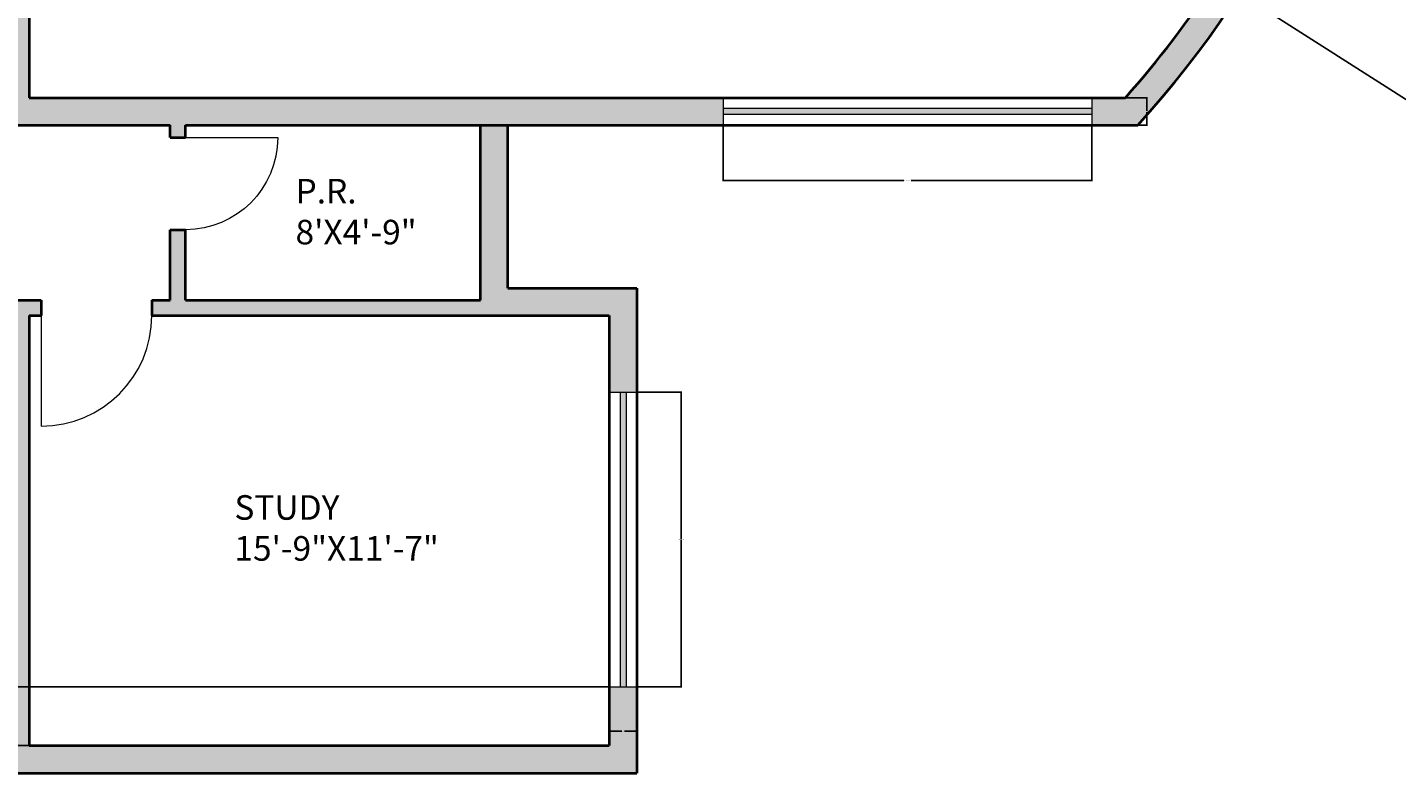
# Model space of a CAD drawing. Units: inches. Extents: x 2330 to 3943, y 1763 to 3461.
# Tile 13 of 40: x 2977 to 3423, y 2300 to 2547. Entities that reach past the tile are written whole.
import ezdxf

# ---------------------------------------------------------------- set-up
doc = ezdxf.new("R2010")
doc.units = ezdxf.units.IN
for name, color, linetype, lineweight in [('A-ANNO-DIMS', 2, 'Continuous', 18), ('A-AREA-IDEN', 7, 'Continuous', 18), ('A-DOOR', 4, 'Continuous', 18), ('A-GLAZ', 4, 'Continuous', 18), ('A-WALL', 7, 'Continuous', 40), ('A-WALL-PATT', 252, 'Continuous', 13), ('L-PLNT', 94, 'Continuous', 13)]:
    doc.layers.add(name, color=color, linetype=linetype, lineweight=lineweight)
doc.styles.get("Standard").update_dxf_attribs({"font": 'arial.ttf'})
doc.dimstyles.get("Standard").update_dxf_attribs({"dimtxt": 0.18, "dimasz": 0.18, "dimexe": 0.18, "dimexo": 0.0625, "dimgap": 0.09, "dimtad": 0, "dimtih": 1, "dimtoh": 1, "dimdec": 4, "dimzin": 0, "dimdsep": 46, "dimtxsty": 'Standard', "dimcen": 0.09, "dimadec": 0, "dimazin": 0, "dimtfac": 1, "dimtdec": 4, "dimtofl": 0, "dimtmove": 0, "dimatfit": 3, "dimfxl": 1, "dimtolj": 1, "dimtzin": 0, "dimarcsym": 0})

# ---------------------------------------------------------------- blocks, each defined once
blk = doc.blocks.new('DOOR-SINGLE-36IN')
blk.add_line((0, 0), (-36, 0))
blk.add_arc((0, 0), 36, 180, 270)
blk = doc.blocks.new('DOOR-SINGLE-30IN')
blk.add_line((0, 0), (0, 30))
blk.add_arc((0, 0), 30, 90, 180)
blk = doc.blocks.new('WINDOW-96IN')
h = blk.add_hatch(color=256)
h.dxf.hatch_style = 1
h.paths.add_polyline_path([(5.5, 96), (3.5, 96), (3.5, 0), (5.5, 0)])
for p, q in [((0, 96), (9, 96)), ((3.5, 96), (3.5, 0)), ((5.5, 96), (5.5, 0)), ((0, 0), (9, 0))]:
    blk.add_line(p, q)
blk = doc.blocks.new('WINDOW-120IN')
h = blk.add_hatch(color=256)
h.dxf.hatch_style = 1
h.paths.add_polyline_path([(120, 5.5), (0, 5.5), (0, 3.5), (120, 3.5)])
for p, q in [((0, 9), (0, 0)), ((120, 9), (120, 0)), ((120, 5.5), (0, 5.5)), ((120, 3.5), (0, 3.5))]:
    blk.add_line(p, q)
blk = doc.blocks.new('*D33')
at = {"layer": 'A-ANNO-DIMS', "color": 0, "lineweight": -2, "transparency": 16777216}
for p, q in [((3203.78, 2514.59), (3203.78, 2496.47)), ((3323.78, 2514.59), (3323.78, 2496.47)), ((3203.96, 2496.65), (3262.59, 2496.65)), ((3323.6, 2496.65), (3264.97, 2496.65))]:
    blk.add_line(p, q, dxfattribs=at)
at = {"layer": 'A-ANNO-DIMS', "color": 0, "transparency": 16777216}
for points in [[(3203.96, 2496.68), (3203.96, 2496.62), (3203.78, 2496.65)], [(3323.6, 2496.68), (3323.6, 2496.62), (3323.78, 2496.65)]]:
    blk.add_solid(points, dxfattribs=at)
at = {"layer": 'Defpoints', "color": 0, "transparency": 16777216}
for p in [(3203.78, 2514.65), (3323.78, 2514.65), (3323.78, 2496.65)]:
    blk.add_point(p, dxfattribs=at)
at = {"layer": 'A-ANNO-DIMS', "color": 0, "transparency": 16777216, "insert": (3263.78, 2496.65), "char_height": 0.18, "attachment_point": 5}
blk.add_mtext('\\A1;WINDOW 120 TYP.', dxfattribs=at)
blk = doc.blocks.new('*D34')
at = {"layer": 'A-ANNO-DIMS', "color": 0, "lineweight": -2, "transparency": 16777216}
for p, q in [((3323.84, 2523.65), (3341.96, 2523.65)), ((3341.78, 2523.47), (3341.78, 2519.33)), ((3341.78, 2514.83), (3341.78, 2518.97)), ((3323.84, 2514.65), (3341.96, 2514.65))]:
    blk.add_line(p, q, dxfattribs=at)
at = {"layer": 'A-ANNO-DIMS', "color": 0, "transparency": 16777216}
for points in [[(3341.75, 2523.47), (3341.81, 2523.47), (3341.78, 2523.65)], [(3341.75, 2514.83), (3341.81, 2514.83), (3341.78, 2514.65)]]:
    blk.add_solid(points, dxfattribs=at)
at = {"layer": 'Defpoints', "color": 0, "transparency": 16777216}
for p in [(3323.78, 2523.65), (3341.78, 2523.65), (3323.78, 2514.65)]:
    blk.add_point(p, dxfattribs=at)
at = {"layer": 'A-ANNO-DIMS', "color": 0, "transparency": 16777216, "insert": (3341.78, 2519.15), "char_height": 0.18, "attachment_point": 5}
blk.add_mtext('\\A1;9 TYP.', dxfattribs=at)
blk = doc.blocks.new('*D35')
at = {"layer": 'A-ANNO-DIMS', "color": 0, "lineweight": -2, "transparency": 16777216}
for p, q in [((3175.72, 2427.7), (3190.24, 2427.7)), ((3190.06, 2427.52), (3190.06, 2379.88)), ((3190.06, 2331.88), (3190.06, 2379.52)), ((3175.72, 2331.7), (3190.24, 2331.7))]:
    blk.add_line(p, q, dxfattribs=at)
at = {"layer": 'A-ANNO-DIMS', "color": 0, "transparency": 16777216}
for points in [[(3190.03, 2427.52), (3190.09, 2427.52), (3190.06, 2427.7)], [(3190.03, 2331.88), (3190.09, 2331.88), (3190.06, 2331.7)]]:
    blk.add_solid(points, dxfattribs=at)
at = {"layer": 'Defpoints', "color": 0, "transparency": 16777216}
for p in [(3175.66, 2427.7), (3190.06, 2427.7), (3175.66, 2331.7)]:
    blk.add_point(p, dxfattribs=at)
at = {"layer": 'A-ANNO-DIMS', "color": 0, "transparency": 16777216, "insert": (3190.06, 2379.7), "char_height": 0.18, "attachment_point": 5}
blk.add_mtext('\\A1;WINDOW 96 TYP.', dxfattribs=at)
blk = doc.blocks.new('*D36')
at = {"layer": 'A-ANNO-DIMS', "color": 0, "lineweight": -2, "transparency": 16777216}
for p, q in [((3166.66, 2331.64), (3166.66, 2317.12)), ((3175.66, 2331.64), (3175.66, 2317.12)), ((3166.84, 2317.3), (3170.7, 2317.3)), ((3175.48, 2317.3), (3171.62, 2317.3))]:
    blk.add_line(p, q, dxfattribs=at)
at = {"layer": 'A-ANNO-DIMS', "color": 0, "transparency": 16777216}
for points in [[(3166.84, 2317.33), (3166.84, 2317.27), (3166.66, 2317.3)], [(3175.48, 2317.33), (3175.48, 2317.27), (3175.66, 2317.3)]]:
    blk.add_solid(points, dxfattribs=at)
at = {"layer": 'Defpoints', "color": 0, "transparency": 16777216}
for p in [(3166.66, 2331.7), (3175.66, 2331.7), (3175.66, 2317.3)]:
    blk.add_point(p, dxfattribs=at)
at = {"layer": 'A-ANNO-DIMS', "color": 0, "transparency": 16777216, "insert": (3171.16, 2317.3), "char_height": 0.18, "attachment_point": 5}
blk.add_mtext('\\A1;9 TYP.', dxfattribs=at)
blk = doc.blocks.new('*D80')
at = {"layer": 'A-ANNO-DIMS', "color": 0, "lineweight": -2, "transparency": 16777216}
for p, q in [((3166.6, 2331.7), (2330.5, 2331.7)), ((2330.68, 2331.52), (2330.68, 2322.36)), ((2330.68, 2312.83), (2330.68, 2321.99)), ((3166.6, 2312.65), (2330.5, 2312.65))]:
    blk.add_line(p, q, dxfattribs=at)
at = {"layer": 'A-ANNO-DIMS', "color": 0, "transparency": 16777216}
for points in [[(2330.65, 2331.52), (2330.71, 2331.52), (2330.68, 2331.7)], [(2330.65, 2312.83), (2330.71, 2312.83), (2330.68, 2312.65)]]:
    blk.add_solid(points, dxfattribs=at)
at = {"layer": 'Defpoints', "color": 0, "transparency": 16777216}
for p in [(2330.68, 2331.7), (3166.66, 2331.7), (3166.66, 2312.65)]:
    blk.add_point(p, dxfattribs=at)
at = {"layer": 'A-ANNO-DIMS', "color": 0, "transparency": 16777216, "insert": (2330.68, 2322.18), "char_height": 0.18, "attachment_point": 5}
blk.add_mtext('\\A1;19.046', dxfattribs=at)
blk = doc.blocks.new('*D98')
at = {"layer": 'A-ANNO-DIMS', "color": 0, "lineweight": -2, "transparency": 16777216}
for p, q in [((3105.6, 2727.69), (3105.78, 2727.69)), ((3105.69, 2727.6), (3105.69, 2727.78)), ((3519.33, 2463.49), (3364.37, 2562.47)), ((3519.51, 2463.49), (3519.33, 2463.49))]:
    blk.add_line(p, q, dxfattribs=at)
at = {"layer": 'A-ANNO-DIMS', "color": 0, "transparency": 16777216}
blk.add_solid([(3364.39, 2562.49), (3364.35, 2562.44), (3364.22, 2562.56)], dxfattribs=at)
at = {"layer": 'Defpoints', "color": 0, "transparency": 16777216}
for p in [(3105.69, 2727.69), (3364.22, 2562.56)]:
    blk.add_point(p, dxfattribs=at)
at = {"layer": 'A-ANNO-DIMS', "color": 0, "transparency": 16777216, "insert": (3520.26, 2463.49), "char_height": 0.18, "attachment_point": 5}
blk.add_mtext('\\A1;3X R306.76', dxfattribs=at)
blk = doc.blocks.new('*D103')
at = {"layer": 'A-ANNO-DIMS', "color": 0, "lineweight": -2, "transparency": 16777216}
for p, q in [((3257.55, 2659.32), (3257.73, 2659.32)), ((3257.64, 2659.23), (3257.64, 2659.41)), ((3257.66, 1763.59), (3257.65, 2099.31)), ((3257.84, 1763.59), (3257.66, 1763.59))]:
    blk.add_line(p, q, dxfattribs=at)
at = {"layer": 'A-ANNO-DIMS', "color": 0, "transparency": 16777216}
blk.add_solid([(3257.68, 2099.31), (3257.62, 2099.31), (3257.65, 2099.49)], dxfattribs=at)
at = {"layer": 'Defpoints', "color": 0, "transparency": 16777216}
for p in [(3257.64, 2659.32), (3257.65, 2099.49)]:
    blk.add_point(p, dxfattribs=at)
at = {"layer": 'A-ANNO-DIMS', "color": 0, "transparency": 16777216, "insert": (3258.58, 1763.59), "char_height": 0.18, "attachment_point": 5}
blk.add_mtext('\\A1;40X R559.8', dxfattribs=at)
blk = doc.blocks.new('*D104')
at = {"layer": 'A-ANNO-DIMS', "color": 0, "lineweight": -2, "transparency": 16777216}
for p, q in [((3257.55, 2659.32), (3257.73, 2659.32)), ((3257.64, 2659.23), (3257.64, 2659.41)), ((3257.66, 1917.19), (3257.65, 2195.31)), ((3257.84, 1917.19), (3257.66, 1917.19))]:
    blk.add_line(p, q, dxfattribs=at)
at = {"layer": 'A-ANNO-DIMS', "color": 0, "transparency": 16777216}
blk.add_solid([(3257.68, 2195.31), (3257.62, 2195.31), (3257.65, 2195.49)], dxfattribs=at)
at = {"layer": 'Defpoints', "color": 0, "transparency": 16777216}
for p in [(3257.64, 2659.32), (3257.65, 2195.49)]:
    blk.add_point(p, dxfattribs=at)
at = {"layer": 'A-ANNO-DIMS', "color": 0, "transparency": 16777216, "insert": (3258.58, 1917.19), "char_height": 0.18, "attachment_point": 5}
blk.add_mtext('\\A1;33X R463.8', dxfattribs=at)

msp = doc.modelspace()

# ---------------------------------------------------------------- hatches: boundary and pattern name
at = {"layer": 'A-WALL-PATT'}
h = msp.add_hatch(color=256, dxfattribs=at)
h.dxf.hatch_style = 1
h.paths.add_polyline_path([(3203.7816, 2523.6524), (2977.6605, 2523.6524), (2977.6605, 2700.6524), (2981.6605, 2700.6524), (2981.6605, 2705.6524), (2977.6605, 2705.6524), (2977.6605, 2733.6524), (2968.6605, 2733.6524), (2968.6605, 2514.6524), (3023.6605, 2514.6524), (3023.6605, 2510.6524), (3028.6605, 2510.6524), (3028.6605, 2514.6524), (3203.7816, 2514.6524)])
h = msp.add_hatch(color=256, dxfattribs=at)
h.dxf.hatch_style = 1
h.paths.add_polyline_path([(3410.1519, 2643.9665), (3401.474, 2646.3527, -0.03078214), (3389.25, 2610.6524), (3277.6605, 2610.6524), (3277.6605, 2605.6524), (3387.1343, 2605.6524, -0.07980087), (3334.7596, 2523.6524), (3323.7816, 2523.6524), (3323.7816, 2514.6524), (3338.7607, 2514.6524, 0.11859459)])
h = msp.add_hatch(color=256, dxfattribs=at)
h.dxf.hatch_style = 1
h.paths.add_polyline_path([(3175.6605, 2461.6524), (3133.6605, 2461.6524), (3133.6605, 2514.6524), (3124.6605, 2514.6524), (3124.6605, 2457.6524), (3028.6605, 2457.6524), (3028.6605, 2480.6524), (3023.6605, 2480.6524), (3023.6605, 2457.6524), (3017.6605, 2457.6524), (3017.6605, 2452.6524), (3166.6605, 2452.6524), (3166.6605, 2427.6982), (3175.6605, 2427.6982)])
h = msp.add_hatch(color=256, dxfattribs=at)
h.dxf.hatch_style = 1
h.paths.add_polyline_path([(2977.6605, 2452.6524), (2981.6605, 2452.6524), (2981.6605, 2457.6524), (2968.6605, 2457.6524), (2855.1605, 2457.6524), (2855.1605, 2448.6524), (2968.6605, 2448.6524), (2968.6605, 2303.6524), (3175.6605, 2303.6524), (3175.6605, 2331.6982), (3166.6605, 2331.6982), (3166.6605, 2312.6524), (2977.6605, 2312.6524)])

# ---------------------------------------------------------------- linework, layer by layer
at = {"layer": 'A-WALL'}
for p, q in [((2977.6605, 2700.6524), (2977.6605, 2523.6524)), ((2977.6605, 2523.6524), (3334.7596, 2523.6524)), ((2968.6605, 2514.6524), (3023.6605, 2514.6524)), ((3023.6605, 2510.6524), (3023.6605, 2514.6524)), ((3028.6605, 2510.6524), (3028.6605, 2514.6524)), ((3028.6605, 2514.6524), (3338.7607, 2514.6524)), ((3124.6605, 2457.6524), (3124.6605, 2514.6524)), ((3133.6605, 2461.6524), (3133.6605, 2514.6524)), ((3023.6605, 2510.6524), (3028.6605, 2510.6524)), ((3023.6605, 2457.6524), (3023.6605, 2480.6524)), ((3023.6605, 2480.6524), (3028.6605, 2480.6524)), ((3028.6605, 2457.6524), (3028.6605, 2480.6524)), ((2968.6605, 2457.6524), (2981.6605, 2457.6524)), ((2981.6605, 2457.6524), (2981.6605, 2452.6524)), ((3017.6605, 2457.6524), (3017.6605, 2452.6524)), ((3017.6605, 2457.6524), (3023.6605, 2457.6524)), ((3028.6605, 2457.6524), (3124.6605, 2457.6524)), ((3133.6605, 2461.6524), (3175.6605, 2461.6524)), ((3175.6605, 2461.6524), (3175.6605, 2303.6524)), ((2977.6605, 2452.6524), (2981.6605, 2452.6524)), ((2977.6605, 2452.6524), (2977.6605, 2312.6524)), ((3017.6605, 2452.6524), (3166.6605, 2452.6524)), ((3166.6605, 2452.6524), (3166.6605, 2312.6524)), ((2977.6605, 2312.6524), (3166.6605, 2312.6524)), ((2968.6605, 2303.6524), (3175.6605, 2303.6524))]:
    msp.add_line(p, q, dxfattribs=at)
for radius, start, end in [(315.7595, 317.571214, 26.95911), (306.7595, 318.307811, 336.558149)]:
    msp.add_arc((3105.6935, 2727.6869), radius, start, end, dxfattribs=at)
at = {"layer": 'L-PLNT'}
msp.add_line((2977.6605, 2359.8307), (2977.8818, 2359.7101), dxfattribs=at)

# ---------------------------------------------------------------- block references
at = {"layer": 'A-DOOR', "extrusion": (0, 0, -1), "zscale": -1, "rotation": 89.99999999999866}
msp.add_blockref('DOOR-SINGLE-30IN', (-3028.6605, 2510.6524), dxfattribs=at)
at = {"layer": 'A-DOOR', "rotation": 90.00000000000072}
msp.add_blockref('DOOR-SINGLE-36IN', (2981.6605, 2452.6524), dxfattribs=at)
at = {"layer": 'A-GLAZ'}
for name, p in [('WINDOW-120IN', (3203.7816, 2514.6524)), ('WINDOW-96IN', (3166.6605, 2331.6982))]:
    msp.add_blockref(name, p, dxfattribs=at)

# ---------------------------------------------------------------- texts
at = {"layer": 'A-AREA-IDEN', "char_height": 8, "attachment_point": 1}
for s, width, insert in [('P.R.\\P8\'X4\'-9"', 58.351217, (3064.4554, 2497.2071)), ('STUDY\\P15\'-9"X11\'-7"', 112.783732, (3044.5545, 2394.1741))]:
    msp.add_mtext_dynamic_manual_height_columns(s, width=width, gutter_width=12.5, heights=[0], dxfattribs=dict(at, insert=insert))

# ---------------------------------------------------------------- dimensions: what is measured, and where the dimension line sits
at = {"layer": 'A-ANNO-DIMS'}
for center, mpoint, text, override, picture, middle in [((3105.6935, 2727.6869), (3364.219, 2562.563), '3X <>', {"dimdec": 2, "dimlfac": 1, "dimrnd": 0, "dimzin": 0, "dimdsep": 46, "dimlunit": 2}, '*D98', (3520.2574, 2463.4886)), ((3257.6403, 2659.3212), (3257.65, 2099.4902), '40X <>', {"dimdec": 1, "dimlfac": 1, "dimrnd": 0, "dimzin": 0, "dimdsep": 46, "dimlunit": 2}, '*D103', (3258.5828, 1763.5916)), ((3257.6403, 2659.3212), (3257.65, 2195.4902), '33X <>', {"dimdec": 1, "dimlfac": 1, "dimrnd": 0, "dimzin": 0, "dimdsep": 46, "dimlunit": 2}, '*D104', (3258.5791, 1917.1916))]:
    dim = msp.add_radius_dim(center=center, mpoint=mpoint, text=text, dimstyle='Standard', override=override, dxfattribs=at)
    dim.commit()
    dim.dimension.update_dxf_attribs({"geometry": picture, "text_midpoint": middle, "dimtype": 164})
for base, p1, p2, text, picture, middle in [((3341.7816, 2523.6524), (3323.7816, 2514.6524), (3323.7816, 2523.6524), '<> TYP.', '*D34', (3341.7816, 2519.1524)), ((3190.0605, 2427.6982), (3175.6605, 2331.6982), (3175.6605, 2427.6982), 'WINDOW <> TYP.', '*D35', (3190.0605, 2379.6982))]:
    dim = msp.add_linear_dim(base=base, p1=p1, p2=p2, angle=90, text=text, dimstyle='Standard', override={"dimdec": 0, "dimlfac": 1, "dimrnd": 0, "dimzin": 0, "dimdsep": 46, "dimlunit": 2}, dxfattribs=at)
    dim.commit()
    dim.dimension.update_dxf_attribs({"geometry": picture, "text_midpoint": middle})
for base, p1, p2, text, picture, middle in [((3323.7816, 2496.6524), (3203.7816, 2514.6524), (3323.7816, 2514.6524), 'WINDOW <> TYP.', '*D33', (3263.7816, 2496.6524)), ((3175.6605, 2317.2982), (3166.6605, 2331.6982), (3175.6605, 2331.6982), '<> TYP.', '*D36', (3171.1605, 2317.2982))]:
    dim = msp.add_linear_dim(base=base, p1=p1, p2=p2, text=text, dimstyle='Standard', override={"dimdec": 0, "dimlfac": 1, "dimrnd": 0, "dimzin": 0, "dimdsep": 46, "dimlunit": 2}, dxfattribs=at)
    dim.commit()
    dim.dimension.update_dxf_attribs({"geometry": picture, "text_midpoint": middle})
dim = msp.add_linear_dim(base=(2330.6824, 2331.6982), p1=(3166.6605, 2312.6524), p2=(3166.6605, 2331.6982), angle=90, dimstyle='Standard', override={"dimdec": 3, "dimlfac": 1, "dimrnd": 0, "dimzin": 0, "dimdsep": 46, "dimlunit": 2}, dxfattribs=at)
dim.commit()
dim.dimension.update_dxf_attribs({"geometry": '*D80', "text_midpoint": (2330.6824, 2322.1753)})

doc.saveas('drawing.dxf')
